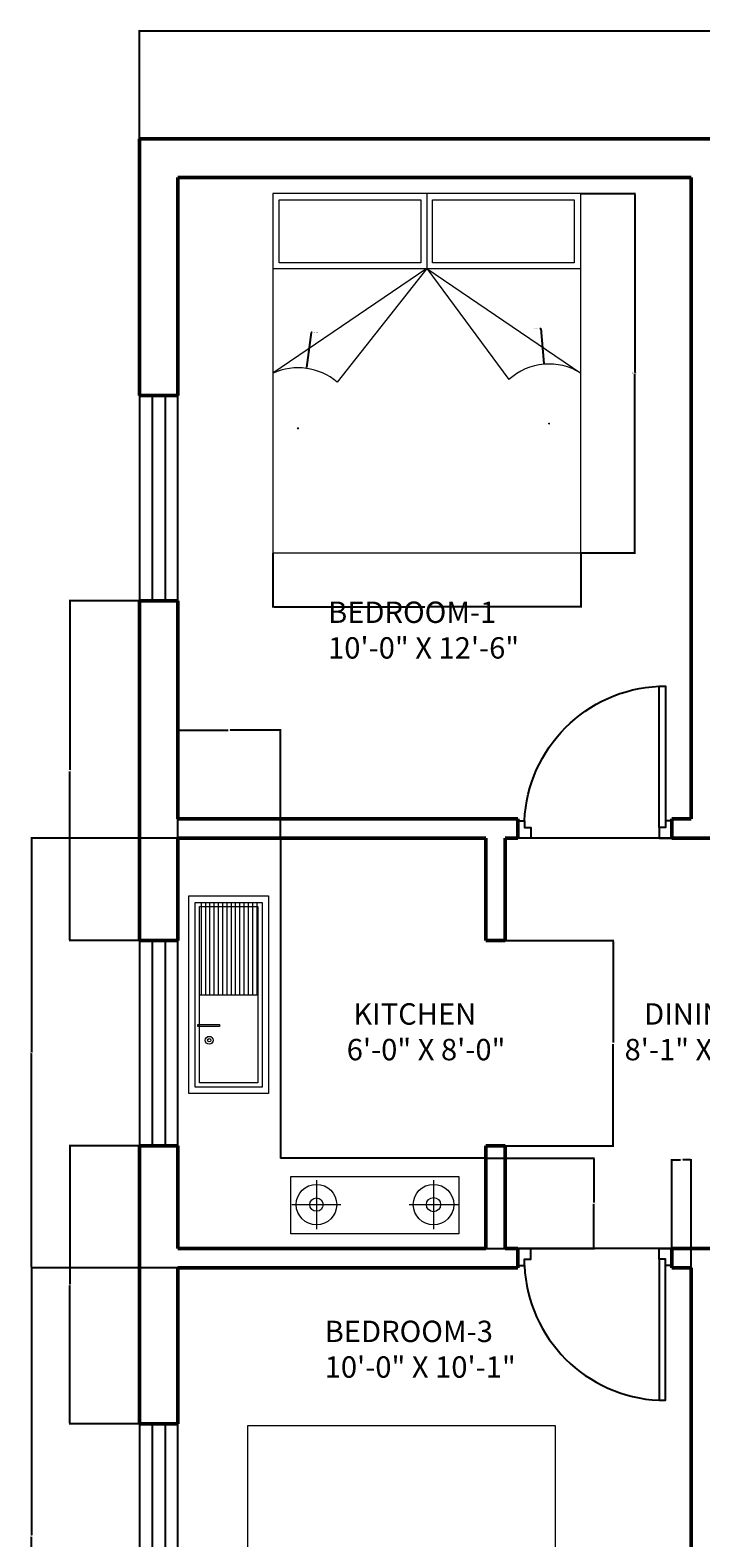
# Model space of a CAD drawing. Units: inches. Extents: x 17078 to 17468, y 5298 to 5853.
# Tile 2 of 3: x 17078 to 17235, y 5500 to 5853. Entities that reach past the tile are written whole.
import ezdxf

# ---------------------------------------------------------------- set-up
doc = ezdxf.new("R2010")
doc.units = ezdxf.units.IN
for name, color, linetype, lineweight in [('A-ANNO-DIMS', 2, 'Continuous', 18), ('A-AREA-IDEN', 7, 'Continuous', 18), ('A-EQPM', 9, 'Continuous', 18), ('A-FLOR-CASE', 9, 'Continuous', 25), ('A-FLOR-FIXT', 9, 'Continuous', 18), ('A-FLOR-FIXT-PATT', 9, 'Continuous', 13), ('door', 30, 'Continuous', 25), ('furniture', 9, 'Continuous', 18), ('wall', 7, 'Continuous', 50), ('window1', 151, 'Continuous', 25)]:
    doc.layers.add(name, color=color, linetype=linetype, lineweight=lineweight)
doc.styles.get("Standard").update_dxf_attribs({"font": 'arial.ttf'})
doc.dimstyles.get("Standard").update_dxf_attribs({"dimtxt": 0.18, "dimasz": 0.18, "dimexe": 0.18, "dimexo": 0.0625, "dimgap": 0.09, "dimtad": 0, "dimtih": 1, "dimtoh": 1, "dimdec": 4, "dimzin": 0, "dimdsep": 46, "dimtxsty": 'Standard', "dimcen": 0.09, "dimadec": 0, "dimazin": 0, "dimtfac": 1, "dimtdec": 4, "dimtofl": 0, "dimtmove": 0, "dimatfit": 3, "dimfxl": 1, "dimtolj": 1, "dimtzin": 0, "dimarcsym": 0})

# ---------------------------------------------------------------- blocks, each defined once
blk = doc.blocks.new('w2')
at = {"layer": 'window1'}
for p, q in [((17539.72, 5675.98), (17539.72, 5627.98)), ((17542.72, 5675.98), (17542.72, 5627.98))]:
    blk.add_line(p, q, dxfattribs=at)
blk.add_lwpolyline([(17536.72, 5627.98), (17545.72, 5627.98), (17545.72, 5675.98), (17536.72, 5675.98)], close=True, dxfattribs=at)
blk = doc.blocks.new('d1')
at = {"layer": 'door'}
blk.add_line((17631.7, 5593.67), (17667.7, 5593.67), dxfattribs=at)
blk.add_lwpolyline([(17633.2, 5596.17), (17634.7, 5596.17), (17634.7, 5629.17), (17633.2, 5629.17)], close=True, dxfattribs=at)
for points in [[(17634.7, 5593.67), (17631.7, 5593.67), (17631.7, 5597.67), (17633.2, 5597.67), (17633.2, 5596.17), (17634.7, 5596.17), (17634.7, 5593.67)], [(17664.7, 5593.67), (17667.7, 5593.67), (17667.7, 5597.67), (17666.2, 5597.67), (17666.2, 5596.17), (17664.7, 5596.17), (17664.7, 5593.67)]]:
    blk.add_lwpolyline(points, dxfattribs=at)
blk.add_arc((17633.2, 5596.17), 33.03, 2.6026, 87.3974, dxfattribs=at)
blk = doc.blocks.new('BED')
at = {"layer": 'furniture'}
for p, q in [((17631.72, 5825.16), (17631.72, 5807.64)), ((17595.72, 5807.64), (17667.72, 5807.64)), ((17631.72, 5807.64), (17595.72, 5783.16)), ((17631.72, 5807.64), (17610.71, 5781.09)), ((17631.72, 5807.64), (17667.72, 5783.16)), ((17631.72, 5807.64), (17650.87, 5781.67))]:
    blk.add_line(p, q, dxfattribs=at)
for points in [[(17595.72, 5741.16), (17667.72, 5741.16), (17667.72, 5825.16), (17595.72, 5825.16)], [(17597.14, 5823.74), (17630.27, 5823.74), (17630.27, 5809), (17597.14, 5809)], [(17633.01, 5823.74), (17666.14, 5823.74), (17666.14, 5809), (17633.01, 5809)]]:
    blk.add_lwpolyline(points, close=True, dxfattribs=at)
for centre, radius, start, end in [((17601.58, 5770.29), 14.15, 49.7949, 114.4561), ((17660.27, 5771.38), 13.94, 57.7012, 132.4176)]:
    blk.add_arc(centre, radius, start, end, dxfattribs=at)
blk = doc.blocks.new('*D19')
at = {"layer": 'A-ANNO-DIMS', "color": 0, "lineweight": -2, "transparency": 16777216}
for p, q in [((17206.82, 5814.72), (17219.53, 5814.72)), ((17219.35, 5814.54), (17219.35, 5772.9)), ((17219.35, 5730.9), (17219.35, 5772.54)), ((17206.82, 5730.72), (17219.53, 5730.72))]:
    blk.add_line(p, q, dxfattribs=at)
at = {"layer": 'A-ANNO-DIMS', "color": 0, "transparency": 16777216}
for points in [[(17219.32, 5814.54), (17219.38, 5814.54), (17219.35, 5814.72)], [(17219.32, 5730.9), (17219.38, 5730.9), (17219.35, 5730.72)]]:
    blk.add_solid(points, dxfattribs=at)
at = {"layer": 'Defpoints', "color": 0, "transparency": 16777216}
for p in [(17206.75, 5814.72), (17219.35, 5814.72), (17206.75, 5730.72)]:
    blk.add_point(p, dxfattribs=at)
at = {"layer": 'A-ANNO-DIMS', "color": 0, "transparency": 16777216, "insert": (17219.35, 5772.72), "char_height": 0.18, "attachment_point": 5}
blk.add_mtext('\\A1;BED 84 TYP.', dxfattribs=at)
blk = doc.blocks.new('*D20')
at = {"layer": 'A-ANNO-DIMS', "color": 0, "lineweight": -2, "transparency": 16777216}
for p, q in [((17134.75, 5730.65), (17134.75, 5717.94)), ((17206.75, 5730.65), (17206.75, 5717.94)), ((17134.93, 5718.12), (17170.23, 5718.12)), ((17206.57, 5718.12), (17171.28, 5718.12))]:
    blk.add_line(p, q, dxfattribs=at)
at = {"layer": 'A-ANNO-DIMS', "color": 0, "transparency": 16777216}
for points in [[(17134.93, 5718.15), (17134.93, 5718.09), (17134.75, 5718.12)], [(17206.57, 5718.15), (17206.57, 5718.09), (17206.75, 5718.12)]]:
    blk.add_solid(points, dxfattribs=at)
at = {"layer": 'Defpoints', "color": 0, "transparency": 16777216}
for p in [(17134.75, 5730.72), (17206.75, 5730.72), (17206.75, 5718.12)]:
    blk.add_point(p, dxfattribs=at)
at = {"layer": 'A-ANNO-DIMS', "color": 0, "transparency": 16777216, "insert": (17170.75, 5718.12), "char_height": 0.18, "attachment_point": 5}
blk.add_mtext('\\A1;72 TYP.', dxfattribs=at)
blk = doc.blocks.new('*D21')
at = {"layer": 'A-ANNO-DIMS', "color": 0, "lineweight": -2, "transparency": 16777216}
for p, q in [((17103.53, 5827.58), (17103.53, 5852.95)), ((17103.71, 5852.77), (17247.24, 5852.77)), ((17391.35, 5852.77), (17247.82, 5852.77)), ((17391.53, 5827.58), (17391.53, 5852.95))]:
    blk.add_line(p, q, dxfattribs=at)
at = {"layer": 'A-ANNO-DIMS', "color": 0, "transparency": 16777216}
for points in [[(17103.71, 5852.8), (17103.71, 5852.74), (17103.53, 5852.77)], [(17391.35, 5852.8), (17391.35, 5852.74), (17391.53, 5852.77)]]:
    blk.add_solid(points, dxfattribs=at)
at = {"layer": 'Defpoints', "color": 0, "transparency": 16777216}
for p in [(17391.53, 5852.77), (17103.53, 5827.52), (17391.53, 5827.52)]:
    blk.add_point(p, dxfattribs=at)
at = {"layer": 'A-ANNO-DIMS', "color": 0, "transparency": 16777216, "insert": (17247.53, 5852.77), "char_height": 0.18, "attachment_point": 5}
blk.add_mtext('\\A1;288', dxfattribs=at)
blk = doc.blocks.new('*D24')
at = {"layer": 'A-ANNO-DIMS', "color": 0, "lineweight": -2, "transparency": 16777216}
for p, q in [((17112.47, 5563.52), (17078.1, 5563.52)), ((17078.28, 5563.34), (17078.28, 5500.95)), ((17078.28, 5438.2), (17078.28, 5500.59)), ((17112.47, 5438.02), (17078.1, 5438.02))]:
    blk.add_line(p, q, dxfattribs=at)
at = {"layer": 'A-ANNO-DIMS', "color": 0, "transparency": 16777216}
for points in [[(17078.25, 5563.34), (17078.31, 5563.34), (17078.28, 5563.52)], [(17078.25, 5438.2), (17078.31, 5438.2), (17078.28, 5438.02)]]:
    blk.add_solid(points, dxfattribs=at)
at = {"layer": 'Defpoints', "color": 0, "transparency": 16777216}
for p in [(17078.28, 5563.52), (17112.53, 5563.52), (17112.53, 5438.02)]:
    blk.add_point(p, dxfattribs=at)
at = {"layer": 'A-ANNO-DIMS', "color": 0, "transparency": 16777216, "insert": (17078.28, 5500.77), "char_height": 0.18, "attachment_point": 5}
blk.add_mtext('\\A1;125.5', dxfattribs=at)
blk = doc.blocks.new('*D25')
at = {"layer": 'A-ANNO-DIMS', "color": 0, "lineweight": -2, "transparency": 16777216}
for p, q in [((17112.47, 5664.02), (17078.1, 5664.02)), ((17078.28, 5663.84), (17078.28, 5613.95)), ((17078.28, 5563.7), (17078.28, 5613.59)), ((17112.47, 5563.52), (17078.1, 5563.52))]:
    blk.add_line(p, q, dxfattribs=at)
at = {"layer": 'A-ANNO-DIMS', "color": 0, "transparency": 16777216}
for points in [[(17078.25, 5663.84), (17078.31, 5663.84), (17078.28, 5664.02)], [(17078.25, 5563.7), (17078.31, 5563.7), (17078.28, 5563.52)]]:
    blk.add_solid(points, dxfattribs=at)
at = {"layer": 'Defpoints', "color": 0, "transparency": 16777216}
for p in [(17078.28, 5664.02), (17112.53, 5664.02), (17112.53, 5563.52)]:
    blk.add_point(p, dxfattribs=at)
at = {"layer": 'A-ANNO-DIMS', "color": 0, "transparency": 16777216, "insert": (17078.28, 5613.77), "char_height": 0.18, "attachment_point": 5}
blk.add_mtext('\\A1;100.5', dxfattribs=at)
blk = doc.blocks.new('*D30')
at = {"layer": 'A-ANNO-DIMS', "color": 0, "lineweight": -2, "transparency": 16777216}
for p, q in [((17112.47, 5592.02), (17087.1, 5592.02)), ((17087.28, 5591.84), (17087.28, 5559.7)), ((17087.28, 5527.2), (17087.28, 5559.34)), ((17112.47, 5527.02), (17087.1, 5527.02))]:
    blk.add_line(p, q, dxfattribs=at)
at = {"layer": 'A-ANNO-DIMS', "color": 0, "transparency": 16777216}
for points in [[(17087.25, 5591.84), (17087.31, 5591.84), (17087.28, 5592.02)], [(17087.25, 5527.2), (17087.31, 5527.2), (17087.28, 5527.02)]]:
    blk.add_solid(points, dxfattribs=at)
at = {"layer": 'Defpoints', "color": 0, "transparency": 16777216}
for p in [(17087.28, 5592.02), (17112.53, 5592.02), (17112.53, 5527.02)]:
    blk.add_point(p, dxfattribs=at)
at = {"layer": 'A-ANNO-DIMS', "color": 0, "transparency": 16777216, "insert": (17087.28, 5559.52), "char_height": 0.18, "attachment_point": 5}
blk.add_mtext('\\A1;65', dxfattribs=at)
blk = doc.blocks.new('*D31')
at = {"layer": 'A-ANNO-DIMS', "color": 0, "lineweight": -2, "transparency": 16777216}
for p, q in [((17112.47, 5719.52), (17087.1, 5719.52)), ((17087.28, 5719.34), (17087.28, 5679.95)), ((17087.28, 5640.2), (17087.28, 5679.59)), ((17112.47, 5640.02), (17087.1, 5640.02))]:
    blk.add_line(p, q, dxfattribs=at)
at = {"layer": 'A-ANNO-DIMS', "color": 0, "transparency": 16777216}
for points in [[(17087.25, 5719.34), (17087.31, 5719.34), (17087.28, 5719.52)], [(17087.25, 5640.2), (17087.31, 5640.2), (17087.28, 5640.02)]]:
    blk.add_solid(points, dxfattribs=at)
at = {"layer": 'Defpoints', "color": 0, "transparency": 16777216}
for p in [(17087.28, 5719.52), (17112.53, 5719.52), (17112.53, 5640.02)]:
    blk.add_point(p, dxfattribs=at)
at = {"layer": 'A-ANNO-DIMS', "color": 0, "transparency": 16777216, "insert": (17087.28, 5679.77), "char_height": 0.18, "attachment_point": 5}
blk.add_mtext('\\A1;79.5', dxfattribs=at)
blk = doc.blocks.new('*D37')
at = {"layer": 'A-ANNO-DIMS', "color": 0, "lineweight": -2, "transparency": 16777216}
for p, q in [((17189.1, 5640.02), (17214.46, 5640.02)), ((17214.28, 5639.84), (17214.28, 5616.2)), ((17214.28, 5592.2), (17214.28, 5615.84)), ((17189.1, 5592.02), (17214.46, 5592.02))]:
    blk.add_line(p, q, dxfattribs=at)
at = {"layer": 'A-ANNO-DIMS', "color": 0, "transparency": 16777216}
for points in [[(17214.25, 5639.84), (17214.31, 5639.84), (17214.28, 5640.02)], [(17214.25, 5592.2), (17214.31, 5592.2), (17214.28, 5592.02)]]:
    blk.add_solid(points, dxfattribs=at)
at = {"layer": 'Defpoints', "color": 0, "transparency": 16777216}
for p in [(17189.03, 5640.02), (17189.03, 5592.02), (17214.28, 5592.02)]:
    blk.add_point(p, dxfattribs=at)
at = {"layer": 'A-ANNO-DIMS', "color": 0, "transparency": 16777216, "insert": (17214.28, 5616.02), "char_height": 0.18, "attachment_point": 5}
blk.add_mtext('\\A1;48', dxfattribs=at)
blk = doc.blocks.new('*D38')
at = {"layer": 'A-ANNO-DIMS', "color": 0, "lineweight": -2, "transparency": 16777216}
for p, q in [((17112.53, 5664.08), (17112.53, 5689.45)), ((17112.71, 5689.27), (17124.31, 5689.27)), ((17136.35, 5689.27), (17124.75, 5689.27)), ((17136.53, 5664.08), (17136.53, 5689.45))]:
    blk.add_line(p, q, dxfattribs=at)
at = {"layer": 'A-ANNO-DIMS', "color": 0, "transparency": 16777216}
for points in [[(17112.71, 5689.3), (17112.71, 5689.24), (17112.53, 5689.27)], [(17136.35, 5689.3), (17136.35, 5689.24), (17136.53, 5689.27)]]:
    blk.add_solid(points, dxfattribs=at)
at = {"layer": 'Defpoints', "color": 0, "transparency": 16777216}
for p in [(17136.53, 5689.27), (17112.53, 5664.02), (17136.53, 5664.02)]:
    blk.add_point(p, dxfattribs=at)
at = {"layer": 'A-ANNO-DIMS', "color": 0, "transparency": 16777216, "insert": (17124.53, 5689.27), "char_height": 0.18, "attachment_point": 5}
blk.add_mtext('\\A1;24', dxfattribs=at)
blk = doc.blocks.new('*D39')
at = {"layer": 'A-ANNO-DIMS', "color": 0, "lineweight": -2, "transparency": 16777216}
for p, q in [((17184.6, 5589.16), (17209.96, 5589.16)), ((17209.78, 5588.98), (17209.78, 5578.77)), ((17209.78, 5568.2), (17209.78, 5578.41)), ((17184.6, 5568.02), (17209.96, 5568.02))]:
    blk.add_line(p, q, dxfattribs=at)
at = {"layer": 'A-ANNO-DIMS', "color": 0, "transparency": 16777216}
for points in [[(17209.75, 5588.98), (17209.81, 5588.98), (17209.78, 5589.16)], [(17209.75, 5568.2), (17209.81, 5568.2), (17209.78, 5568.02)]]:
    blk.add_solid(points, dxfattribs=at)
at = {"layer": 'Defpoints', "color": 0, "transparency": 16777216}
for p in [(17184.53, 5589.16), (17184.53, 5568.02), (17209.78, 5568.02)]:
    blk.add_point(p, dxfattribs=at)
at = {"layer": 'A-ANNO-DIMS', "color": 0, "transparency": 16777216, "insert": (17209.78, 5578.59), "char_height": 0.18, "attachment_point": 5}
blk.add_mtext('\\A1;21.137', dxfattribs=at)
blk = doc.blocks.new('*D42')
at = {"layer": 'A-ANNO-DIMS', "color": 0, "lineweight": -2, "transparency": 16777216}
for p, q in [((17228.03, 5563.58), (17228.03, 5588.95)), ((17228.21, 5588.77), (17230.03, 5588.77)), ((17232.35, 5588.77), (17230.54, 5588.77)), ((17232.53, 5563.58), (17232.53, 5588.95))]:
    blk.add_line(p, q, dxfattribs=at)
at = {"layer": 'A-ANNO-DIMS', "color": 0, "transparency": 16777216}
for points in [[(17228.21, 5588.8), (17228.21, 5588.74), (17228.03, 5588.77)], [(17232.35, 5588.8), (17232.35, 5588.74), (17232.53, 5588.77)]]:
    blk.add_solid(points, dxfattribs=at)
at = {"layer": 'Defpoints', "color": 0, "transparency": 16777216}
for p in [(17232.53, 5588.77), (17228.03, 5563.52), (17232.53, 5563.52)]:
    blk.add_point(p, dxfattribs=at)
at = {"layer": 'A-ANNO-DIMS', "color": 0, "transparency": 16777216, "insert": (17230.28, 5588.77), "char_height": 0.18, "attachment_point": 5}
blk.add_mtext('\\A1;4.5', dxfattribs=at)
blk = doc.blocks.new('*D45')
at = {"layer": 'A-ANNO-DIMS', "color": 0, "lineweight": -2, "transparency": 16777216}
for p, q in [((17143.71, 5782.26), (17142.57, 5774.03)), ((17143.89, 5782.26), (17143.71, 5782.26)), ((17140.52, 5759.84), (17140.7, 5759.84)), ((17140.61, 5759.75), (17140.61, 5759.93))]:
    blk.add_line(p, q, dxfattribs=at)
at = {"layer": 'A-ANNO-DIMS', "color": 0, "transparency": 16777216}
blk.add_solid([(17142.54, 5774.04), (17142.6, 5774.03), (17142.55, 5773.85)], dxfattribs=at)
at = {"layer": 'Defpoints', "color": 0, "transparency": 16777216}
for p in [(17142.55, 5773.85), (17140.61, 5759.84)]:
    blk.add_point(p, dxfattribs=at)
at = {"layer": 'A-ANNO-DIMS', "color": 0, "transparency": 16777216, "insert": (17144.64, 5782.26), "char_height": 0.18, "attachment_point": 5}
blk.add_mtext('\\A1;3X R14.147', dxfattribs=at)
blk = doc.blocks.new('*D46')
at = {"layer": 'A-ANNO-DIMS', "color": 0, "lineweight": -2, "transparency": 16777216}
for p, q in [((17197.16, 5783.15), (17197.34, 5783.15)), ((17197.34, 5783.15), (17198.06, 5775)), ((17199.22, 5760.94), (17199.4, 5760.94)), ((17199.31, 5760.85), (17199.31, 5761.03))]:
    blk.add_line(p, q, dxfattribs=at)
at = {"layer": 'A-ANNO-DIMS', "color": 0, "transparency": 16777216}
blk.add_solid([(17198.09, 5775), (17198.03, 5775), (17198.08, 5774.82)], dxfattribs=at)
at = {"layer": 'Defpoints', "color": 0, "transparency": 16777216}
for p in [(17198.08, 5774.82), (17199.31, 5760.94)]:
    blk.add_point(p, dxfattribs=at)
at = {"layer": 'A-ANNO-DIMS', "color": 0, "transparency": 16777216, "insert": (17196.42, 5783.15), "char_height": 0.18, "attachment_point": 5}
blk.add_mtext('\\A1;3X R13.937', dxfattribs=at)

msp = doc.modelspace()

# ---------------------------------------------------------------- hatches: boundary and pattern name
at = {"layer": 'A-FLOR-FIXT-PATT'}
h = msp.add_hatch(dxfattribs=at)
h.set_pattern_fill('ANSI31', color=256, scale=0.314961, angle=45, style=0)
h.paths.add_polyline_path([(17117.5717, 5627.3519), (17131.2025, 5627.3519), (17131.2025, 5648.971), (17117.5717, 5648.971)])

# ---------------------------------------------------------------- linework, layer by layer
at = {"layer": 'A-EQPM'}
for p, q in [((17144.9172, 5584.018), (17144.9172, 5572.5543)), ((17172.283, 5584.018), (17172.283, 5572.5543)), ((17139.1853, 5578.2862), (17150.6491, 5578.2862)), ((17166.5512, 5578.2862), (17178.0149, 5578.2862))]:
    msp.add_line(p, q, dxfattribs=at)
msp.add_lwpolyline([(17138.9235, 5584.8265), (17178.1978, 5584.8265), (17178.1978, 5571.4307), (17138.9235, 5571.4307)], close=True, dxfattribs=at)
for centre, radius in [((17144.9172, 5578.2862), 4.7319), ((17172.283, 5578.2862), 4.7319), ((17144.9172, 5578.2862), 1.5697), ((17172.283, 5578.2862), 1.6707)]:
    msp.add_circle(centre, radius, dxfattribs=at)
at = {"layer": 'A-FLOR-CASE'}
for p, q in [((17136.534, 5664.02), (17136.534, 5589.1569)), ((17184.534, 5589.1569), (17136.534, 5589.1569)), ((17184.534, 5589.1569), (17184.534, 5592.02))]:
    msp.add_line(p, q, dxfattribs=at)
at = {"layer": 'A-FLOR-FIXT'}
msp.add_line((17117.5717, 5627.3519), (17131.2025, 5627.3519), dxfattribs=at)
for points in [[(17115.0717, 5650.471), (17133.7025, 5650.471), (17133.7025, 5604.2327), (17115.0717, 5604.2327)], [(17116.5717, 5648.971), (17132.2025, 5648.971), (17132.2025, 5605.7327), (17116.5717, 5605.7327)], [(17117.5717, 5647.971), (17131.2025, 5647.971), (17131.2025, 5606.7327), (17117.5717, 5606.7327)], [(17122.2366, 5620.4103), (17122.2366, 5619.9297), (17117.1648, 5619.9297), (17117.1648, 5620.4103)]]:
    msp.add_lwpolyline(points, close=True, dxfattribs=at)
for radius in [0.912, 0.3839]:
    msp.add_circle((17119.8348, 5616.7243), radius, dxfattribs=at)
at = {"layer": 'wall'}
for p, q in [((17391.534, 5827.52), (17103.534, 5827.52)), ((17103.534, 5827.52), (17103.534, 5767.52)), ((17112.534, 5818.52), (17112.534, 5767.52)), ((17232.534, 5818.52), (17112.534, 5818.52)), ((17232.534, 5818.52), (17232.534, 5668.52)), ((17112.534, 5767.52), (17103.534, 5767.52)), ((17112.534, 5719.52), (17103.534, 5719.52)), ((17103.534, 5719.52), (17103.534, 5640.02)), ((17112.534, 5719.52), (17112.534, 5668.52)), ((17192.034, 5668.52), (17112.534, 5668.52)), ((17192.034, 5668.52), (17192.034, 5664.02)), ((17232.534, 5668.52), (17228.034, 5668.52)), ((17228.034, 5668.52), (17228.034, 5664.02)), ((17112.534, 5664.02), (17112.534, 5640.02)), ((17184.534, 5664.02), (17112.534, 5664.02)), ((17184.534, 5664.02), (17184.534, 5640.02)), ((17192.034, 5664.02), (17189.034, 5664.02)), ((17189.034, 5664.02), (17189.034, 5640.02)), ((17241.534, 5664.02), (17228.034, 5664.02)), ((17112.534, 5640.02), (17103.534, 5640.02)), ((17184.534, 5640.02), (17189.034, 5640.02)), ((17112.534, 5592.02), (17103.534, 5592.02)), ((17103.534, 5592.02), (17103.534, 5527.02)), ((17112.534, 5592.02), (17112.534, 5568.02)), ((17184.534, 5592.02), (17189.034, 5592.02)), ((17184.534, 5592.02), (17184.534, 5568.02)), ((17189.034, 5592.02), (17189.034, 5568.02)), ((17184.534, 5568.02), (17112.534, 5568.02)), ((17192.034, 5568.02), (17189.034, 5568.02)), ((17192.034, 5568.02), (17192.034, 5563.52)), ((17237.034, 5568.02), (17228.034, 5568.02)), ((17228.034, 5568.02), (17228.034, 5563.52)), ((17112.534, 5563.52), (17112.534, 5527.02)), ((17192.034, 5563.52), (17112.534, 5563.52)), ((17232.534, 5563.52), (17228.034, 5563.52)), ((17232.534, 5563.52), (17232.534, 5442.52)), ((17112.534, 5527.02), (17103.534, 5527.02))]:
    msp.add_line(p, q, dxfattribs=at)

# ---------------------------------------------------------------- block references
at = {"layer": 'door', "xscale": -1}
msp.add_blockref('d1', (34859.7309, 70.3471), dxfattribs=at)
at = {"layer": 'door', "rotation": 180}
msp.add_blockref('d1', (34859.7309, 11161.6929), dxfattribs=at)
at = {"layer": 'furniture'}
msp.add_blockref('BED', (-460.9664, -10.4456), dxfattribs=at)
at = {"layer": 'furniture', "rotation": 180}
msp.add_blockref('BED', (34796.4989, 11267.683), dxfattribs=at)
at = {"layer": 'window1'}
for p in [(-433.1828, 91.541), (-433.1828, -35.959), (-433.1828, -148.959)]:
    msp.add_blockref('w2', p, dxfattribs=at)

# ---------------------------------------------------------------- texts
at = {"layer": 'A-AREA-IDEN', "char_height": 5, "attachment_point": 1}
for s, insert in [('BEDROOM-1\\P10\'-0" X 12\'-6"', (17147.6327, 5719.3173)), (' KITCHEN\\P6\'-0" X 8\'-0"', (17151.9926, 5625.3725)), ('   DINING\\P8\'-1" X 8\'-0"', (17216.9513, 5625.3725)), ('BEDROOM-3\\P10\'-0" X 10\'-1"', (17146.8369, 5551.1394))]:
    msp.add_mtext_dynamic_manual_height_columns(s, width=48.964, gutter_width=12.5, heights=[0], dxfattribs=dict(at, insert=insert))

# ---------------------------------------------------------------- dimensions: what is measured, and where the dimension line sits
at = {"layer": 'A-ANNO-DIMS'}
for base, p1, p2, override, picture, middle in [((17391.534, 5852.77), (17103.534, 5827.52), (17391.534, 5827.52), {"dimdec": 0, "dimlfac": 1, "dimrnd": 0, "dimzin": 0, "dimdsep": 46, "dimlunit": 2}, '*D21', (17247.534, 5852.77)), ((17136.534, 5689.27), (17112.534, 5664.02), (17136.534, 5664.02), {"dimdec": 0, "dimlfac": 1, "dimrnd": 0, "dimzin": 0, "dimdsep": 46, "dimlunit": 2}, '*D38', (17124.534, 5689.27)), ((17232.534, 5588.77), (17228.034, 5563.52), (17232.534, 5563.52), {"dimdec": 1, "dimlfac": 1, "dimrnd": 0, "dimzin": 0, "dimdsep": 46, "dimlunit": 2}, '*D42', (17230.284, 5588.77))]:
    dim = msp.add_linear_dim(base=base, p1=p1, p2=p2, dimstyle='Standard', override=override, dxfattribs=at)
    dim.commit()
    dim.dimension.update_dxf_attribs({"geometry": picture, "text_midpoint": middle})
dim = msp.add_linear_dim(base=(17219.3536, 5814.7174), p1=(17206.7536, 5730.7174), p2=(17206.7536, 5814.7174), angle=90, text='BED <> TYP.', dimstyle='Standard', override={"dimdec": 0, "dimlfac": 1, "dimrnd": 0, "dimzin": 0, "dimdsep": 46, "dimlunit": 2}, dxfattribs=at)
dim.commit()
dim.dimension.update_dxf_attribs({"geometry": '*D19', "text_midpoint": (17219.3536, 5772.7174)})
for center, mpoint, picture, middle in [((17199.3064, 5760.9366), (17198.077, 5774.8196), '*D46', (17196.4163, 5783.1494)), ((17140.6105, 5759.8395), (17142.549, 5773.8533), '*D45', (17144.6352, 5782.2616))]:
    dim = msp.add_radius_dim(center=center, mpoint=mpoint, text='3X <>', dimstyle='Standard', override={"dimdec": 3, "dimlfac": 1, "dimrnd": 0, "dimzin": 0, "dimdsep": 46, "dimlunit": 2}, dxfattribs=at)
    dim.commit()
    dim.dimension.update_dxf_attribs({"geometry": picture, "text_midpoint": middle, "dimtype": 164})
dim = msp.add_linear_dim(base=(17206.7536, 5718.1174), p1=(17134.7536, 5730.7174), p2=(17206.7536, 5730.7174), text='<> TYP.', dimstyle='Standard', override={"dimdec": 0, "dimlfac": 1, "dimrnd": 0, "dimzin": 0, "dimdsep": 46, "dimlunit": 2}, dxfattribs=at)
dim.commit()
dim.dimension.update_dxf_attribs({"geometry": '*D20', "text_midpoint": (17170.7536, 5718.1174)})
for base, p1, p2, angle, override, picture, middle in [((17087.284, 5719.52), (17112.534, 5640.02), (17112.534, 5719.52), 90, {"dimdec": 1, "dimlfac": 1, "dimrnd": 0, "dimzin": 0, "dimdsep": 46, "dimlunit": 2}, '*D31', (17087.284, 5679.77)), ((17078.284, 5664.02), (17112.534, 5563.52), (17112.534, 5664.02), 90, {"dimdec": 1, "dimlfac": 1, "dimrnd": 0, "dimzin": 0, "dimdsep": 46, "dimlunit": 2}, '*D25', (17078.284, 5613.77)), ((17214.284, 5592.02), (17189.034, 5640.02), (17189.034, 5592.02), 270, {"dimdec": 0, "dimlfac": 1, "dimrnd": 0, "dimzin": 0, "dimdsep": 46, "dimlunit": 2}, '*D37', (17214.284, 5616.02)), ((17087.284, 5592.02), (17112.534, 5527.02), (17112.534, 5592.02), 90, {"dimdec": 0, "dimlfac": 1, "dimrnd": 0, "dimzin": 0, "dimdsep": 46, "dimlunit": 2}, '*D30', (17087.284, 5559.52)), ((17209.784, 5568.02), (17184.534, 5589.1569), (17184.534, 5568.02), 270, {"dimdec": 3, "dimlfac": 1, "dimrnd": 0, "dimzin": 0, "dimdsep": 46, "dimlunit": 2}, '*D39', (17209.784, 5578.5884)), ((17078.284, 5563.52), (17112.534, 5438.02), (17112.534, 5563.52), 90, {"dimdec": 1, "dimlfac": 1, "dimrnd": 0, "dimzin": 0, "dimdsep": 46, "dimlunit": 2}, '*D24', (17078.284, 5500.77))]:
    dim = msp.add_linear_dim(base=base, p1=p1, p2=p2, angle=angle, dimstyle='Standard', override=override, dxfattribs=at)
    dim.commit()
    dim.dimension.update_dxf_attribs({"geometry": picture, "text_midpoint": middle})

doc.saveas('drawing.dxf')
